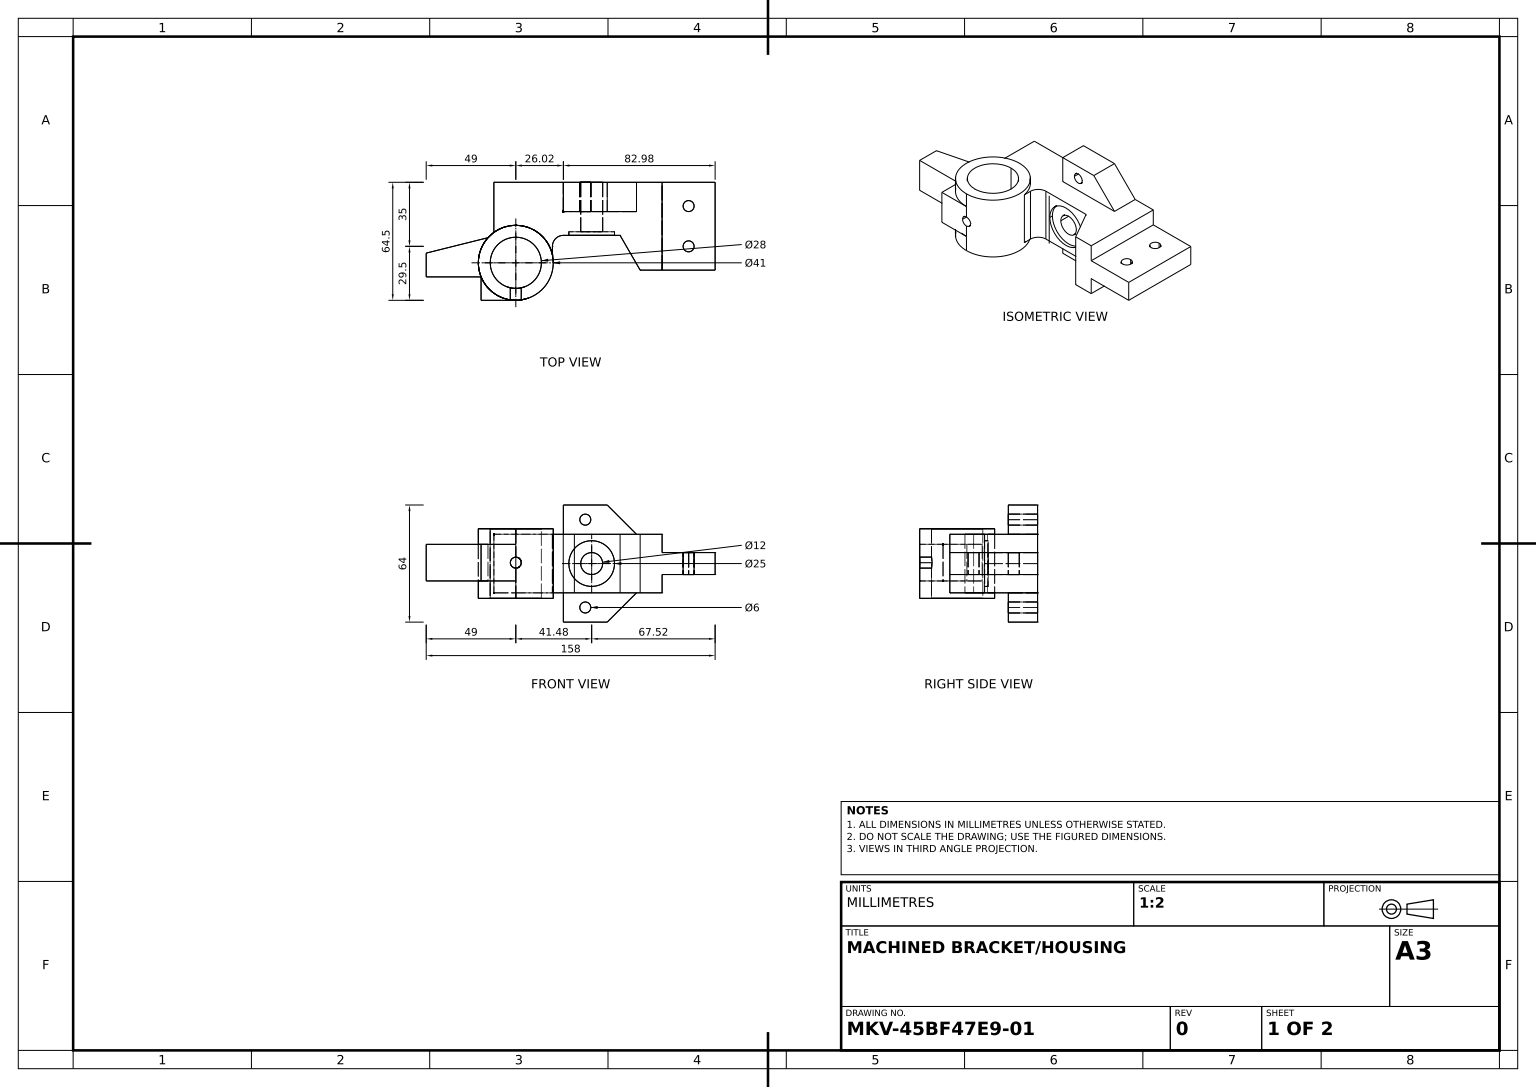
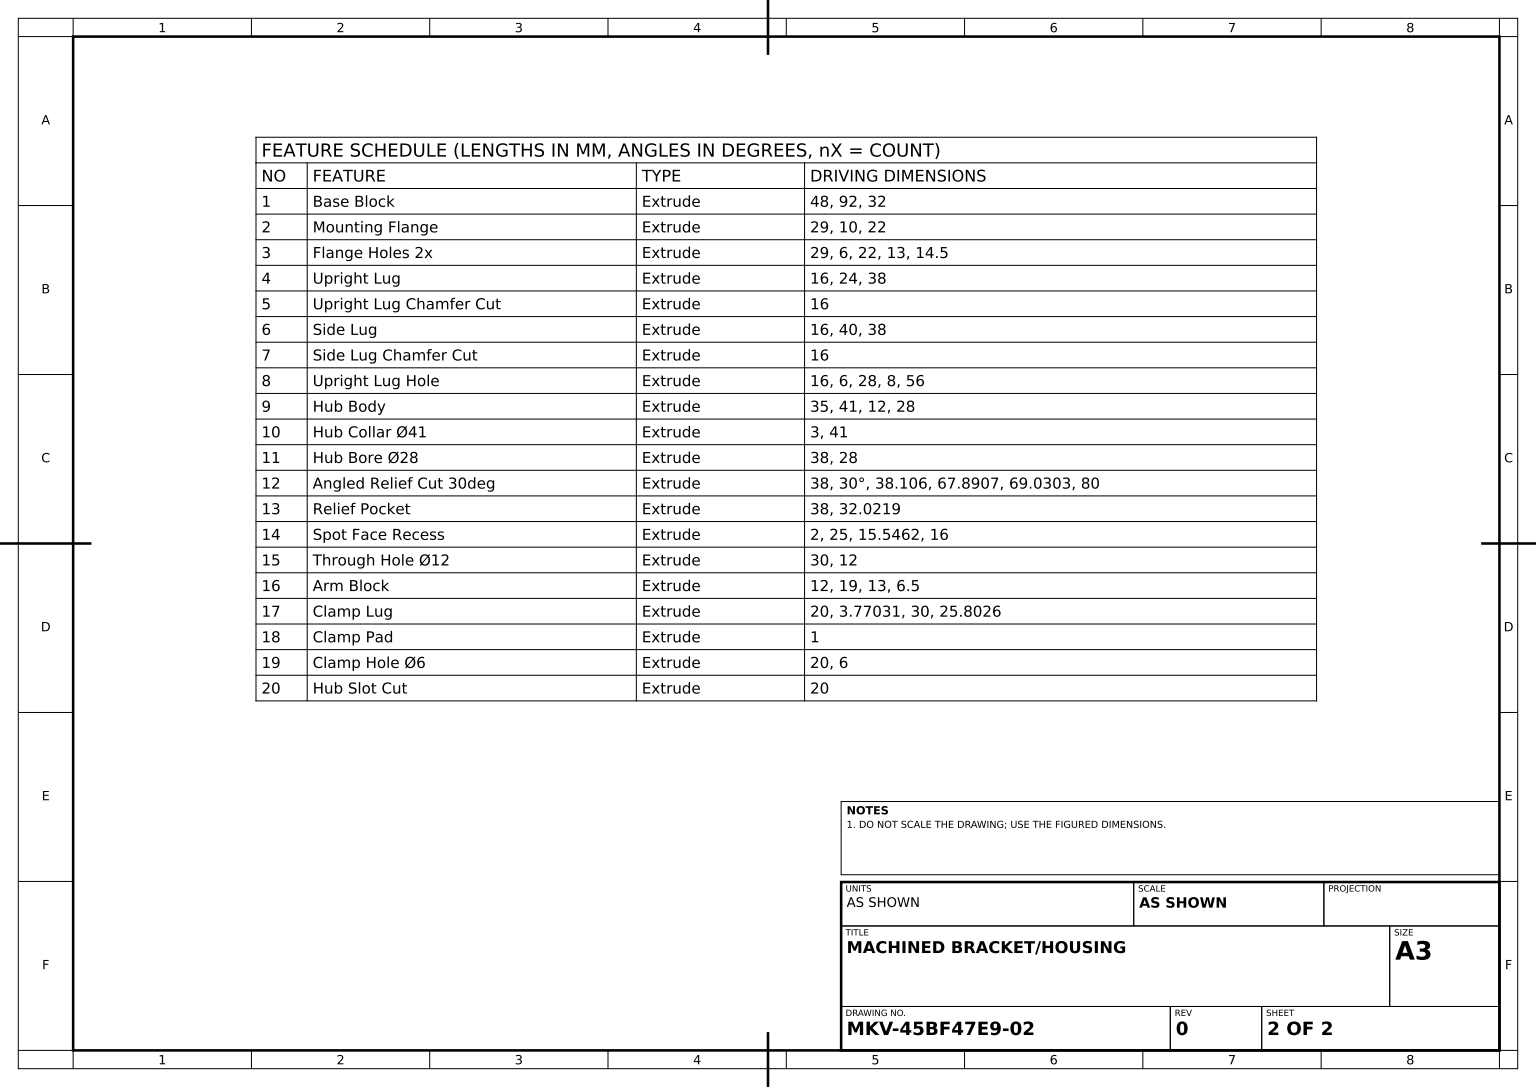
from build123d import *

# Parameters (mm, degrees)
BASE_BLOCK_SKETCH_W           = 92
BASE_BLOCK_SKETCH_H           = 32
BASE_BLOCK_DEPTH              = 48
MOUNTING_FLANGE_SKETCH_W      = 48
MOUNTING_FLANGE_SKETCH_H      = 12.000000000000002
MOUNTING_FLANGE_DEPTH         = 29
FLANGE_HOLES_SKETCH_R         = 2.999999999999994
FLANGE_HOLES_SKETCH_R_2       = 2.9999999999999947
FLANGE_HOLES_2X_DEPTH         = 29
UPRIGHT_LUG_DEPTH             = 16
UPRIGHT_LUG_CHAMFER_CUT_DEPTH = 16
SIDE_LUG_DEPTH                = 16
SIDE_LUG_CHAMFER_CUT_DEPTH    = 16
UPRIGHT_LUG_HOLE_SKETCH_R     = 3.0000000000000018
UPRIGHT_LUG_HOLE_SKETCH_R_2   = 3.000000000000001
UPRIGHT_LUG_HOLE_DEPTH        = 16
HUB_BODY_DEPTH                = 35
HUB_START                     = 3
HUB_COLLAR_SKETCH_R           = 20.5
HUB_COLLAR_41_DEPTH           = 3
HUB_BORE_SKETCH_R             = 13.999999999999996
HUB_BORE_28_DEPTH             = 38
ANGLED_RELIEF_CUT_30DEG_DEPTH = 38
RELIEF_POCKET_DEPTH           = 38
SPOT_FACE_SKETCH_R            = 12.500000000000002
SPOT_FACE_RECESS_DEPTH        = 2
THROUGH_HOLE_SKETCH_R         = 6.000000000000003
THROUGH_HOLE_12_DEPTH         = 30
ARM_BLOCK_SKETCH_W            = 12.999999999999993
ARM_BLOCK_SKETCH_H            = 19.000000000000004
ARM_BLOCK_DEPTH               = 19
CLAMP_LUG_DEPTH               = 20
CLAMP_PAD_DEPTH               = 1
CLAMP_HOLE_SKETCH_R           = 3.0000000000000004
CLAMP_HOLE_6_DEPTH            = 20
HUB_SLOT_CUT_DEPTH            = 20


with BuildPart() as part:
    # Base Block Sketch → Base Block (new body)
    with BuildSketch(Plane.XY):
        with Locations((46, 16)):
            Rectangle(BASE_BLOCK_SKETCH_W, BASE_BLOCK_SKETCH_H)
    extrude(amount=BASE_BLOCK_DEPTH)

    # Mounting Flange Sketch → Mounting Flange (add)
    with BuildSketch(Plane(origin=(92, 0, 0), x_dir=(0, 0, -1), z_dir=(1, 0, 0))):
        with Locations((-24, 16)):
            Rectangle(MOUNTING_FLANGE_SKETCH_W, MOUNTING_FLANGE_SKETCH_H)
    extrude(amount=MOUNTING_FLANGE_DEPTH)

    # Flange Holes Sketch → Flange Holes 2x (cut)
    with BuildSketch(Plane.XZ.offset(-9.999999999999998)):
        with Locations(Location((106.5, 13, 0), (0, 0, 270))):
            Circle(FLANGE_HOLES_SKETCH_R)
        with Locations(Location((106.5, 34.99999999999999, 0), (0, 0, 270))):
            Circle(FLANGE_HOLES_SKETCH_R_2)
    extrude(amount=-FLANGE_HOLES_2X_DEPTH, mode=Mode.SUBTRACT)

    # Upright Lug Sketch → Upright Lug (add)
    with BuildSketch(Plane.XZ):
        Polygon((38, 0), (62, 0), (78, 0), (78, 16), (62, 16), (38, 16), align=None)
    extrude(amount=UPRIGHT_LUG_DEPTH)

    # Upright Lug Chamfer Sketch → Upright Lug Chamfer Cut (cut)
    with BuildSketch(Plane.XY.offset(16)):
        Polygon((78, -16), (62, -16), (78, 0), align=None)
    extrude(amount=-UPRIGHT_LUG_CHAMFER_CUT_DEPTH, mode=Mode.SUBTRACT)

    # Side Lug Sketch → Side Lug (add)
    with BuildSketch(Plane(origin=(0, 32, 0), x_dir=(1, 0, 0), z_dir=(0, 1, 0))):
        Polygon((38, 0), (62, 0), (78, 0), (78, -16), (62, -16), (38, -16), align=None)
    extrude(amount=SIDE_LUG_DEPTH)

    # Side Lug Chamfer Sketch → Side Lug Chamfer Cut (cut)
    with BuildSketch(Plane.XY.offset(16)):
        Polygon((78, 48), (62, 48), (78, 32), align=None)
    extrude(amount=-SIDE_LUG_CHAMFER_CUT_DEPTH, mode=Mode.SUBTRACT)

    # Upright Lug Hole Sketch → Upright Lug Hole (cut)
    with BuildSketch(Plane.XY.offset(16)):
        with Locations((50, 40)):
            Circle(UPRIGHT_LUG_HOLE_SKETCH_R)
        with Locations((50, -8)):
            Circle(UPRIGHT_LUG_HOLE_SKETCH_R_2)
    extrude(amount=-UPRIGHT_LUG_HOLE_DEPTH, mode=Mode.SUBTRACT)

    # Hub Body Sketch → Hub Body (add)
    with BuildSketch(Plane.XZ):
        with BuildLine():
            ThreePointArc((3.3573e-13, 27.379229861405094), (21.334077351297417, 25.748287751556113), (32.5, 43.99999999999999))
            ThreePointArc((32.5, 44), (32.4012544943822, 46.009680336633146), (32.10596926288294, 48.00000000000083))
            Line((32.10596926288278, 48), (0, 48))
            Line((0, 48), (0, 27.379229861404976))
        make_face()
        with BuildLine():
            Line((0, 48), (32.10596926288278, 48))
            ThreePointArc((32.10596926288294, 48.00000000000083), (0.9216100131877187, 61.24874706464494), (3.3573e-13, 27.379229861405094))
            Line((0, 27.379229861404976), (0, 48))
        make_face()
    extrude(amount=-HUB_BODY_DEPTH)

    # Hub Collar Sketch → Hub Collar Ø41 (add)
    with BuildSketch(Plane.XZ.offset(HUB_START)):
        with Locations(Location((11.999999999999998, 44, 0), (0, 0, 270))):
            Circle(HUB_COLLAR_SKETCH_R)
    extrude(amount=-HUB_COLLAR_41_DEPTH)

    # Hub Bore Sketch → Hub Bore Ø28 (cut)
    with BuildSketch(Plane.XZ.offset(3)):
        with Locations(Location((11.999999999999998, 44, 0), (0, 0, 270))):
            Circle(HUB_BORE_SKETCH_R)
    extrude(amount=-HUB_BORE_28_DEPTH, mode=Mode.SUBTRACT)

    # Angled Relief Sketch → Angled Relief Cut 30deg (cut)
    with BuildSketch(Plane.XZ):
        Polygon((69.03034488539707, 29.00000000000001), (79.99999999999999, 48), (38.10596926288314, 48), (38.1059692628831, 29), (67.89066123526882, 29), align=None)
    extrude(amount=-ANGLED_RELIEF_CUT_30DEG_DEPTH, mode=Mode.SUBTRACT)

    # Relief Pocket Sketch → Relief Pocket (cut)
    with BuildSketch(Plane.XZ):
        with BuildLine():
            Line((32.052589846453245, 39.74046476127714), (32.021949545440904, 34.99941169508152))
            ThreePointArc((32.021949545440904, 34.99941169508152), (33.74970667402833, 30.786581192003514), (37.93792982799573, 29.00000000000004))
            Line((37.93792982799573, 29), (38.1059692628831, 29))
            Line((38.1059692628831, 29), (38.10596926288314, 48))
            Line((38.10596926288314, 48), (32.1059692628831, 48))
            ThreePointArc((32.10596926288309, 48), (32.499571898565115, 43.8675161309467), (32.0525898464532, 39.74046476127714))
        make_face()
    extrude(amount=-RELIEF_POCKET_DEPTH, mode=Mode.SUBTRACT)

    # Spot Face Sketch → Spot Face Recess (cut)
    with BuildSketch(Plane.XY.offset(29)):
        with Locations((53.48413735669789, 16)):
            Circle(SPOT_FACE_SKETCH_R)
    extrude(amount=-SPOT_FACE_RECESS_DEPTH, mode=Mode.SUBTRACT)

    # Through Hole Sketch → Through Hole Ø12 (cut)
    with BuildSketch(Plane.XY.offset(27.000000000000004)):
        with Locations((53.48413735669789, 16)):
            Circle(THROUGH_HOLE_SKETCH_R)
    extrude(amount=-THROUGH_HOLE_12_DEPTH, mode=Mode.SUBTRACT)

    # Arm Block Sketch → Arm Block (add)
    with BuildSketch(Plane(origin=(12, 0, 0), x_dir=(0, 0, -1), z_dir=(1, 0, 0))):
        with Locations((-58, 16)):
            Rectangle(ARM_BLOCK_SKETCH_W, ARM_BLOCK_SKETCH_H)
    extrude(amount=-ARM_BLOCK_DEPTH)

    # Clamp Lug Sketch → Clamp Lug (add)
    with BuildSketch(Plane.XZ.offset(-6.499999999999999)):
        with BuildLine():
            Line((-6.999999999999999, 51.69740215917034), (-37, 51.69740215917034))
            Line((-37, 51.69740215917034), (-37, 38.697402159170345))
            Line((-37, 38.697402159170345), (-3.229691527211141, 30.277518592251866))
            ThreePointArc((-3.229691527211141, 30.277518592251866), (-8.189621059274332, 40.446241217681404), (-6.999999999999999, 51.69740215917034))
        make_face()
    extrude(amount=-CLAMP_LUG_DEPTH)

    # Clamp Pad Sketch → Clamp Pad (add)
    with BuildSketch(Plane(origin=(0, 25.5, 0), x_dir=(1, 0, 0), z_dir=(0, 1, 0))):
        with BuildLine():
            Line((-6.999999999999999, -51.69740215917034), (-6.999999999999999, -64.5))
            Line((-6.999999999999999, -64.5), (11.999999999999998, -64.5))
            ThreePointArc((11.999999999999998, -64.5), (0.5445808514701636, -61.00068740173455), (-6.999999999999999, -51.69740215917034))
        make_face()
    extrude(amount=CLAMP_PAD_DEPTH)

    # Clamp Hole Sketch → Clamp Hole Ø6 (cut)
    with BuildSketch(Plane.XY.offset(64.5)):
        with Locations(Location((12, 16.5, 0), (0, 0, 90))):
            Circle(CLAMP_HOLE_SKETCH_R)
    extrude(amount=-CLAMP_HOLE_6_DEPTH, mode=Mode.SUBTRACT)

    # Hub Slot Sketch → Hub Slot Cut (cut)
    with BuildSketch(Plane.XZ.offset(-6.499999999999999)):
        with BuildLine():
            Line((12, 51.50000000000001), (12, 57.99999999999999))
            ThreePointArc((12, 57.99999999999999), (5.254631218383986, 56.26784414638529), (0.17840958246311683, 51.50000000000001))
            Line((0.17840958246311683, 51.50000000000001), (12, 51.50000000000001))
        make_face()
    extrude(amount=-HUB_SLOT_CUT_DEPTH, mode=Mode.SUBTRACT)


solid = part.part
